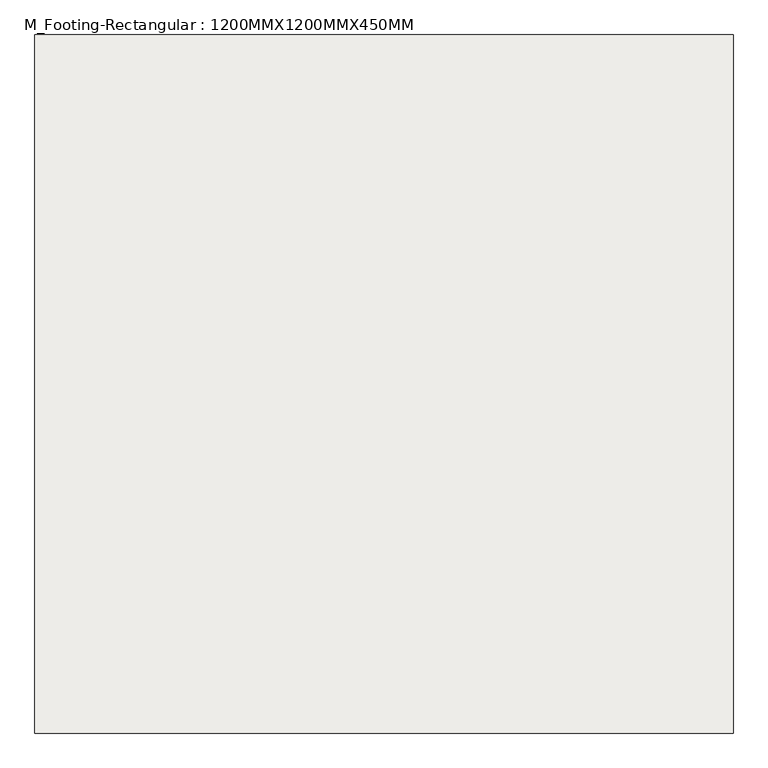
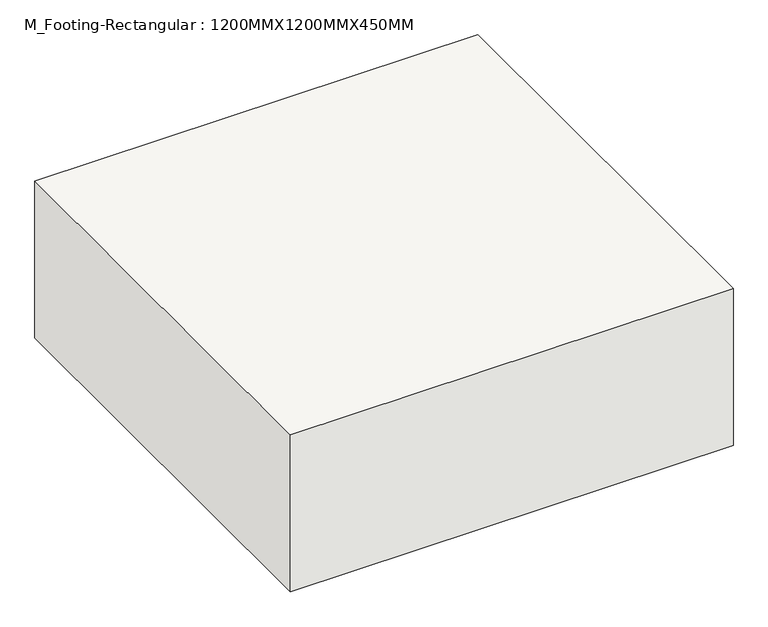
"""IFC4 building model written with IfcOpenShell, lengths in millimetres: slab geometry, M_Footing-Rectangular : 1200MMX1200MMX450MM."""

from ifc_helpers import new_model, si_unit, frame, origin, place, context, project, spatial, polyline, outline, extrude, source, transform, mapped, element, save


def m_footing_rectangular_1200mmx1200mmx450mm_1789818b(model_context):
    return source(origin(), model_context, "Body", "SweptSolid", [
        extrude(outline(polyline([(600.0, 600.0), (600.0, -600.0), (-600.0, -600.0), (-600.0, 600.0), (600.0, 600.0)])), frame((0.0, 0.0, -450.0), z_axis=(0.0, 0.0, 1.0), x_axis=(1.0, 0.0, 0.0)), (0.0, 0.0, 1.0), 450.0),
    ])


if __name__ == "__main__":
    model = new_model("IFC4")
    model_context = context("Model", 3, world=origin())
    ifc_project = project(units=[si_unit("LENGTHUNIT", "METRE", prefix="MILLI")], contexts=[model_context])
    site = spatial("IfcSite", under=ifc_project)
    building = spatial("IfcBuilding", under=site)
    placement = place(None, origin())
    m_footing_rectangular_1200mmx1200mmx450mm_shape = m_footing_rectangular_1200mmx1200mmx450mm_1789818b(model_context)
    element("IfcSlab", 1, ObjectType="M_Footing-Rectangular : 1200MMX1200MMX450MM", at=placement, inside=building, context=model_context, shape_type="MappedRepresentation", body=[
        mapped(m_footing_rectangular_1200mmx1200mmx450mm_shape, transform((0.0, 0.0, 0.0), x_axis=(1.0, 0.0, 0.0), y_axis=(0.0, 1.0, 0.0), z_axis=(0.0, 0.0, 1.0))),
    ])
    save(model, "model.ifc")

# Revit data of these elements
# Type "M_Footing-Rectangular : 1200MMX1200MMX450MM"
#   Width = 1200 mm
#   Length = 1200 mm
#   Foundation Thickness = 450 mm
#   Structural Material [instance default] = Concrete, Cast-in-Place gray
#   Assembly Code = ""
# Element 1 (IfcSlab, "M_Footing-Rectangular : 1200MMX1200MMX450MM")
#   Materials on its faces: "Concrete, Cast-in-Place gray"
# Materials
#   "Concrete, Cast-in-Place gray": class "Concrete", colour RGB 192 192 192, transparency 0, Description = "Cast-in-place concrete", Cost = 0
